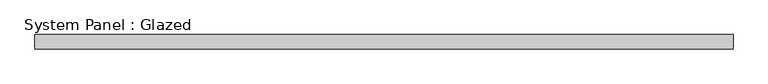
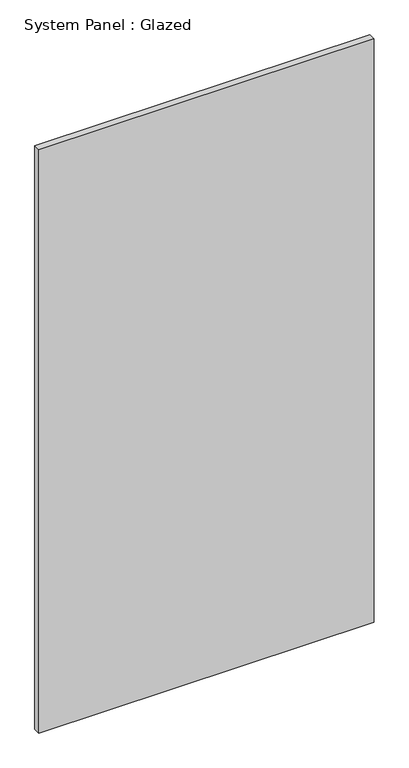
"""IFC4 building model written with IfcOpenShell, lengths in millimetres: plate geometry, System Panel : Glazed."""

from ifc_helpers import new_model, si_unit, origin, origin_with_axes, place, context, project, spatial, polyline, outline, extrude, source, transform, mapped, element, save


def system_panel_glazed_4edfead3(model_context):
    return source(origin(), model_context, "Body", "SweptSolid", [
        extrude(outline(polyline([(628.6499999, 19.05), (-628.6499999, 19.05), (-628.6499999, 44.45), (628.6499999, 44.45), (628.6499999, 19.05)])), origin_with_axes(), (0.0, 0.0, 1.0), 2311.4),
    ])


if __name__ == "__main__":
    model = new_model("IFC4")
    model_context = context("Model", 3, world=origin())
    ifc_project = project(units=[si_unit("LENGTHUNIT", "METRE", prefix="MILLI")], contexts=[model_context])
    site = spatial("IfcSite", under=ifc_project)
    building = spatial("IfcBuilding", under=site)
    placement = place(None, origin())
    system_panel_glazed_shape = system_panel_glazed_4edfead3(model_context)
    element("IfcPlate", 1, ObjectType="System Panel : Glazed", at=placement, inside=building, context=model_context, shape_type="MappedRepresentation", body=[
        mapped(system_panel_glazed_shape, transform((0.0, 0.0, 0.0), x_axis=(1.0, 0.0, 0.0), y_axis=(0.0, 1.0, 0.0), z_axis=(0.0, 0.0, 1.0))),
    ])
    save(model, "model.ifc")

# Revit data of these elements
# Type "System Panel : Glazed"
#   Construction Type Id = "GSP4R"
#   Analytic Construction = "1/8 in Pilkington single glazing"
#   Visual Light Transmittance = 0.9
#   Solar Heat Gain Coefficient = 0.86
#   Heat Transfer Coefficient (U) = 1.18115 BTU/(h·ft²·°F)
#   Define Thermal Properties by = 1
# Element 1 (IfcPlate, "System Panel : Glazed")
#   Materials on its faces: "Glass"
# Materials
#   "Glass": class "Glass", colour RGB 0 128 192, transparency 0.75, Description = "Soda Lime Glass", Cost = 0
